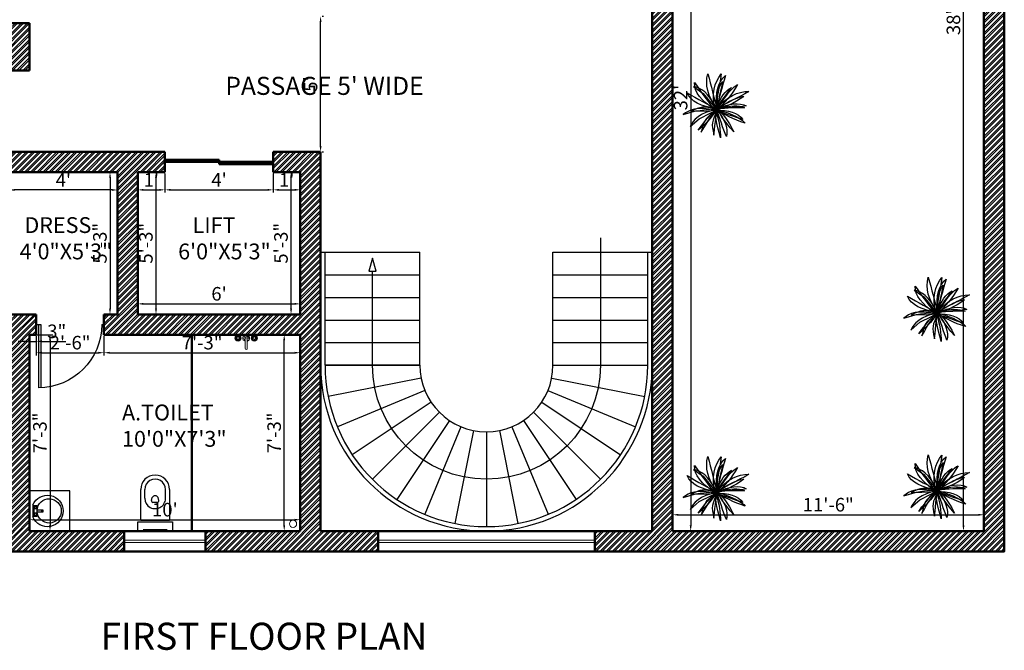
# Model space of a CAD drawing. Units: inches. Extents: x 3590 to 5167, y 65 to 1917.
# Tile 11 of 100: x 4644 to 5080, y 65 to 345. Entities that reach past the tile are written whole.
import ezdxf

# ---------------------------------------------------------------- set-up
doc = ezdxf.new("R2010")
doc.units = ezdxf.units.IN
for name, color, linetype, lineweight in [('A-ANNO-DIMS', 2, 'Continuous', 18), ('A-ANNO-TEXT', 7, 'Continuous', 25), ('A-AREA-IDEN', 7, 'Continuous', 18), ('A-DOOR', 3, 'Continuous', 25), ('A-FLOR-FIXT', 8, 'Continuous', 18), ('A-FLOR-STRS', 7, 'Continuous', 25), ('A-GLAZ', 4, 'Continuous', 18), ('A-WALL', 7, 'Continuous', 50), ('A-WALL-PATT', 251, 'Continuous', 13), ('L-PLNT', 94, 'Continuous', 18)]:
    doc.layers.add(name, color=color, linetype=linetype, lineweight=lineweight)
doc.layers.add('DIENHOA', color=3, linetype='Continuous')
doc.layers.add('SANTEH', color=7, linetype='Continuous')
doc.styles.get("Standard").update_dxf_attribs({"font": 'arial.ttf'})
doc.dimstyles.new('ISO-25', dxfattribs={"dimtxt": 9, "dimasz": 2.5, "dimexe": 1.25, "dimexo": 0.625, "dimtad": 1, "dimdec": 1, "dimlunit": 3, "dimtxsty": 'Standard', "dimcen": 2.5, "dimadec": 0, "dimazin": 0, "dimtfac": 1, "dimtdec": 1, "dimtmove": 0, "dimatfit": 3, "dimfxl": 1, "dimarcsym": 0})

# ---------------------------------------------------------------- blocks, each defined once
blk = doc.blocks.new('*U163')
blk.add_line((-21, 0), (21, 0))
blk = doc.blocks.new('*U162')
at = {"layer": 'A-FLOR-STRS', "color": 0, "linetype": 'ByBlock', "lineweight": -2, "transparency": 16777216}
for p, rotation in [((4076.01, 1459), 89.99999999999982), ((4066.16, 1458.03), 101.2499999999998), ((4085.86, 1458.03), 78.7499999999998), ((4056.69, 1455.15), 112.4999999999998), ((4095.34, 1455.15), 67.4999999999998), ((4047.96, 1450.49), 123.7499999999997), ((4104.07, 1450.49), 56.24999999999984), ((4040.3, 1444.21), 134.9999999999996), ((4111.72, 1444.21), 44.99999999999992), ((4034.02, 1436.56), 146.2499999999996), ((4118, 1436.56), 33.74999999999991), ((4029.36, 1427.82), 157.4999999999995), ((4122.67, 1427.82), 22.49999999999996), ((4026.48, 1418.35), 168.7499999999995), ((4125.54, 1418.35), 11.25), ((4025.51, 1408.5), 180)]:
    blk.add_blockref('*U163', p, dxfattribs=dict(at, rotation=rotation))
blk.add_blockref('*U163', (4126.51, 1408.5), dxfattribs=at)
blk = doc.blocks.new('D2')
for p, q in [((1, 0), (1, 28)), ((2, 0), (2, 27.98)), ((0, 0), (2, 0)), ((29, 0), (30, 0))]:
    blk.add_line(p, q)
at = {"ltscale": 0.5}
blk.add_arc((1, 0), 28, 0, 90, dxfattribs=at)
blk = doc.blocks.new('Cay03_mb')
at = {"layer": 'DIENHOA'}
for p, q in [((79, 504), (119, 555)), ((119, 555), (166, 599)), ((166, 599), (142, 519)), ((-365, 390), (-414, 403)), ((-414, 403), (-240, 278)), ((-315, 371), (-365, 390)), ((-264, 343), (-315, 371)), ((10, 295), (25, 374)), ((25, 374), (49, 444)), ((49, 444), (79, 504)), ((97, 366), (76, 291)), ((119, 442), (97, 366)), ((142, 519), (119, 442)), ((-211, 305), (-264, 343)), ((-240, 278), (-88, 95)), ((-158, 252), (-211, 305)), ((-104, 184), (-158, 252)), ((-50, 98), (-104, 184)), ((0, 105), (2, 206)), ((2, 206), (10, 295)), ((56, 216), (37, 142)), ((76, 291), (56, 216)), ((147, 144), (219, 200)), ((219, 200), (291, 243)), ((364, 193), (290, 155)), ((291, 243), (363, 275)), ((363, 275), (437, 297)), ((438, 231), (364, 193)), ((437, 297), (511, 310)), ((512, 271), (438, 231)), ((511, 310), (586, 314)), ((586, 314), (512, 271)), ((-345, 5), (-400, -17)), ((-299, 20), (-345, 5)), ((-255, 27), (-299, 20)), ((-208, 28), (-255, 27)), ((-153, 22), (-208, 28)), ((-83, 10), (-153, 22)), ((-88, 95), (5, -8)), ((5, -8), (-83, 10)), ((5, -8), (-50, 98)), ((5, -8), (0, 105)), ((5, -8), (76, 75)), ((20, 68), (5, -8)), ((75, 36), (5, -8)), ((5, -8), (100, 18)), ((46, 1), (5, -8)), ((37, 142), (20, 68)), ((97, 7), (46, 1)), ((145, 77), (75, 36)), ((76, 75), (147, 144)), ((155, 12), (97, 7)), ((100, 18), (182, 37)), ((217, 117), (145, 77)), ((220, 15), (155, 12)), ((182, 37), (253, 49)), ((290, 155), (217, 117)), ((289, 17), (220, 15)), ((253, 49), (315, 54)), ((362, 19), (289, 17)), ((315, 54), (369, 53)), ((436, 19), (362, 19)), ((369, 53), (419, 47)), ((419, 47), (465, 35)), ((510, 19), (436, 19)), ((465, 35), (510, 19)), ((-400, -17), (-468, -48)), ((-468, -48), (-376, -38)), ((-376, -38), (-295, -28)), ((-295, -28), (-226, -19)), ((-226, -19), (-166, -11)), ((-216, -236), (-166, -174)), ((-166, -11), (-114, -6)), ((-166, -174), (-120, -122)), ((-120, -122), (-80, -80)), ((-75, -127), (-118, -181)), ((-114, -6), (-69, -3)), ((-80, -80), (-45, -46)), ((-33, -69), (-75, -127)), ((-69, -3), (-30, -3)), ((-45, -46), (-17, -22)), ((5, -8), (-33, -69)), ((-30, -3), (5, -8)), ((-17, -22), (5, -8)), ((5, -8), (57, -73)), ((26, -64), (5, -8)), ((5, -8), (113, -40)), ((53, -42), (5, -8)), ((47, -126), (26, -64)), ((69, -191), (47, -126)), ((107, -76), (53, -42)), ((57, -73), (100, -139)), ((100, -139), (136, -204)), ((166, -110), (107, -76)), ((113, -40), (207, -74)), ((229, -143), (166, -110)), ((207, -74), (290, -108)), ((296, -175), (229, -143)), ((290, -108), (359, -141)), ((367, -205), (296, -175)), ((359, -141), (417, -174)), ((417, -174), (463, -204)), ((-330, -387), (-271, -307)), ((-291, -355), (-330, -387)), ((-250, -318), (-291, -355)), ((-271, -307), (-216, -236)), ((-206, -276), (-250, -318)), ((-162, -231), (-206, -276)), ((-118, -181), (-162, -231)), ((91, -257), (69, -191)), ((113, -322), (91, -257)), ((135, -386), (113, -322)), ((136, -204), (163, -268)), ((163, -268), (181, -330)), ((181, -330), (190, -390)), ((442, -233), (367, -205)), ((519, -258), (442, -233)), ((463, -204), (496, -232)), ((496, -232), (519, -258)), ((158, -445), (135, -386)), ((180, -499), (158, -445)), ((190, -446), (180, -499)), ((190, -390), (190, -446))]:
    blk.add_line(p, q, dxfattribs=at)
for points in [[(24, -5), (-41, 82), (-92, 167), (-130, 249), (-156, 330), (-170, 408), (-175, 484), (-170, 559), (-157, 633)], [(-157, 633), (-132, 551), (-111, 470), (-90, 389), (-70, 309), (-49, 229), (-27, 150), (-3, 72), (24, -5)], [(-16, -27), (-38, 80), (-49, 178), (-49, 269), (-39, 353), (-19, 430), (9, 501), (45, 567), (88, 629)], [(88, 629), (75, 544), (61, 461), (46, 379), (31, 298), (16, 217), (3, 136), (-8, 55), (-16, -27)], [(-396, 474), (-348, 406), (-301, 339), (-254, 275), (-208, 212), (-162, 151), (-115, 91), (-66, 32), (-16, -27)], [(-16, -27), (-108, 39), (-187, 102), (-252, 163), (-305, 224), (-345, 285), (-374, 347), (-390, 409), (-396, 474)], [(273, 387), (228, 329), (182, 270), (138, 212), (97, 156), (60, 103), (28, 55), (2, 11), (-16, -27)], [(-16, -27), (21, 64), (57, 140), (91, 203), (125, 255), (160, 297), (195, 332), (233, 362), (273, 387)], [(24, -5), (20, 93), (20, 177), (25, 249), (34, 310), (47, 363), (65, 409), (87, 452), (113, 492)], [(113, 492), (96, 420), (79, 347), (64, 276), (50, 208), (38, 145), (30, 87), (25, 36), (24, -5)], [(384, 437), (342, 368), (298, 302), (253, 239), (206, 181), (159, 127), (113, 78), (68, 34), (24, -5)], [(24, -5), (80, 92), (134, 176), (186, 248), (234, 309), (279, 357), (319, 395), (355, 421), (384, 437)], [(-530, 290), (-458, 248), (-388, 208), (-319, 169), (-251, 131), (-183, 95), (-115, 60), (-46, 26), (24, -5)], [(24, -5), (-87, 15), (-185, 40), (-270, 68), (-344, 101), (-406, 140), (-457, 184), (-499, 233), (-530, 290)], [(497, 224), (429, 178), (362, 137), (294, 99), (227, 66), (162, 37), (100, 11), (40, -10), (-16, -27)], [(-16, -27), (75, 38), (160, 92), (237, 136), (307, 170), (368, 195), (420, 213), (463, 222), (497, 224)], [(-16, -27), (-134, -5), (-235, 5), (-322, 5), (-396, -5), (-459, -22), (-512, -46), (-558, -74), (-598, -105)], [(24, -5), (99, 30), (173, 57), (245, 77), (313, 88), (378, 92), (438, 87), (493, 74), (541, 52)], [(541, 52), (484, 43), (421, 35), (354, 28), (285, 21), (216, 14), (148, 8), (83, 2), (24, -5)], [(-598, -105), (-393, -44), (-155, -37), (-16, -27)], [(-472, -320), (-310, -179), (-98, -73), (24, -5)], [(24, -5), (-92, -35), (-188, -68), (-267, -105), (-330, -145), (-380, -187), (-418, -231), (-448, -275), (-472, -320)], [(-276, -424), (-227, -345), (-186, -276), (-150, -216), (-119, -164), (-91, -120), (-66, -82), (-41, -52), (-16, -27)], [(-16, -27), (-85, -86), (-137, -133), (-176, -173), (-204, -210), (-226, -249), (-243, -295), (-258, -352), (-276, -424)], [(24, -5), (-14, -88), (-41, -153), (-60, -205), (-70, -251), (-73, -295), (-69, -344), (-60, -402), (-45, -475)], [(-45, -475), (-34, -383), (-25, -303), (-18, -233), (-12, -173), (-6, -121), (2, -77), (11, -39), (24, -5)], [(76, -524), (49, -428), (27, -342), (9, -264), (-4, -196), (-12, -138), (-17, -90), (-18, -53), (-16, -27)], [(478, -192), (422, -176), (361, -157), (298, -135), (232, -113), (167, -89), (102, -67), (41, -45), (-16, -27)], [(-16, -27), (67, -27), (146, -33), (219, -45), (286, -63), (346, -87), (398, -117), (443, -152), (478, -192)], [(-16, -27), (8, -95), (29, -163), (44, -231), (56, -296), (65, -359), (71, -419), (74, -474), (76, -524)], [(316, -418), (251, -343), (195, -273), (147, -210), (106, -154), (74, -105), (50, -63), (33, -30), (24, -5)], [(24, -5), (75, -57), (122, -111), (164, -165), (203, -219), (237, -273), (267, -324), (294, -373), (316, -418)]]:
    blk.add_lwpolyline(points, dxfattribs=at)
blk = doc.blocks.new('*D179')
at = {"layer": 'A-ANNO-DIMS', "color": 0, "lineweight": -2, "transparency": 16777216}
for p, q in [((4639.27, 276.43), (4639.27, 267.91)), ((4687.27, 276.43), (4687.27, 267.91)), ((4684.77, 269.16), (4641.77, 269.16))]:
    blk.add_line(p, q, dxfattribs=at)
at = {"layer": 'A-ANNO-DIMS', "color": 0, "transparency": 16777216}
for points in [[(4641.77, 269.57), (4641.77, 268.74), (4639.27, 269.16)], [(4684.77, 269.57), (4684.77, 268.74), (4687.27, 269.16)]]:
    blk.add_solid(points, dxfattribs=at)
at = {"layer": 'Defpoints', "color": 0, "transparency": 16777216}
for p in [(4639.27, 277.06), (4687.27, 277.06), (4639.27, 269.16)]:
    blk.add_point(p, dxfattribs=at)
at = {"layer": 'A-ANNO-DIMS', "color": 0, "transparency": 16777216, "insert": (4663.27, 272.78), "char_height": 6, "attachment_point": 5}
blk.add_mtext("4'", dxfattribs=at)
blk = doc.blocks.new('*D180')
at = {"layer": 'A-ANNO-DIMS', "color": 0, "lineweight": -2, "transparency": 16777216}
for p, q in [((4686.65, 277.06), (4682.7, 277.06)), ((4683.95, 274.56), (4683.95, 216.56)), ((4686.65, 214.06), (4682.7, 214.06))]:
    blk.add_line(p, q, dxfattribs=at)
at = {"layer": 'A-ANNO-DIMS', "color": 0, "transparency": 16777216}
for points in [[(4683.54, 274.56), (4684.37, 274.56), (4683.95, 277.06)], [(4683.54, 216.56), (4684.37, 216.56), (4683.95, 214.06)]]:
    blk.add_solid(points, dxfattribs=at)
at = {"layer": 'Defpoints', "color": 0, "transparency": 16777216}
for p in [(4687.27, 277.06), (4683.95, 214.06), (4687.27, 214.06)]:
    blk.add_point(p, dxfattribs=at)
at = {"layer": 'A-ANNO-DIMS', "color": 0, "transparency": 16777216, "insert": (4680.26, 245.56), "char_height": 6, "attachment_point": 5, "rotation": 90}
blk.add_mtext('5\'-3"', dxfattribs=at)
blk = doc.blocks.new('*D257')
at = {"layer": 'A-ANNO-DIMS', "color": 0, "lineweight": -2, "transparency": 16777216}
for p, q in [((4645.77, 202.08), (4643.27, 202.08)), ((4648.27, 204.43), (4648.27, 200.83)), ((4648.27, 202.08), (4651.27, 202.08)), ((4651.27, 204.43), (4651.27, 200.83)), ((4653.77, 202.08), (4664.42, 202.08))]:
    blk.add_line(p, q, dxfattribs=at)
at = {"layer": 'A-ANNO-DIMS', "color": 0, "transparency": 16777216}
for points in [[(4645.77, 202.49), (4645.77, 201.66), (4648.27, 202.08)], [(4653.77, 202.49), (4653.77, 201.66), (4651.27, 202.08)]]:
    blk.add_solid(points, dxfattribs=at)
at = {"layer": 'Defpoints', "color": 0, "transparency": 16777216}
for p in [(4648.27, 205.06), (4651.27, 205.06), (4651.27, 202.08)]:
    blk.add_point(p, dxfattribs=at)
at = {"layer": 'A-ANNO-DIMS', "color": 0, "transparency": 16777216, "insert": (4660.35, 205.77), "char_height": 6, "attachment_point": 5}
blk.add_mtext('3"', dxfattribs=at)
blk = doc.blocks.new('*D258')
at = {"layer": 'A-ANNO-DIMS', "color": 0, "lineweight": -2, "transparency": 16777216}
for p, q in [((4651.27, 204.43), (4651.27, 195.81)), ((4681.27, 204.43), (4681.27, 195.81)), ((4653.77, 197.06), (4678.77, 197.06))]:
    blk.add_line(p, q, dxfattribs=at)
at = {"layer": 'A-ANNO-DIMS', "color": 0, "transparency": 16777216}
for points in [[(4653.77, 197.48), (4653.77, 196.65), (4651.27, 197.06)], [(4678.77, 197.48), (4678.77, 196.65), (4681.27, 197.06)]]:
    blk.add_solid(points, dxfattribs=at)
at = {"layer": 'Defpoints', "color": 0, "transparency": 16777216}
for p in [(4651.27, 205.06), (4681.27, 205.06), (4681.27, 197.06)]:
    blk.add_point(p, dxfattribs=at)
at = {"layer": 'A-ANNO-DIMS', "color": 0, "transparency": 16777216, "insert": (4666.27, 200.75), "char_height": 6, "attachment_point": 5}
blk.add_mtext('2\'-6"', dxfattribs=at)
blk = doc.blocks.new('*D259')
at = {"layer": 'A-ANNO-DIMS', "color": 0, "lineweight": -2, "transparency": 16777216}
for p, q in [((4681.27, 204.43), (4681.27, 195.81)), ((4768.27, 204.43), (4768.27, 195.81)), ((4683.77, 197.06), (4765.77, 197.06))]:
    blk.add_line(p, q, dxfattribs=at)
at = {"layer": 'A-ANNO-DIMS', "color": 0, "transparency": 16777216}
for points in [[(4683.77, 197.48), (4683.77, 196.65), (4681.27, 197.06)], [(4765.77, 197.48), (4765.77, 196.65), (4768.27, 197.06)]]:
    blk.add_solid(points, dxfattribs=at)
at = {"layer": 'Defpoints', "color": 0, "transparency": 16777216}
for p in [(4681.27, 205.06), (4768.27, 205.06), (4768.27, 197.06)]:
    blk.add_point(p, dxfattribs=at)
at = {"layer": 'A-ANNO-DIMS', "color": 0, "transparency": 16777216, "insert": (4724.77, 200.75), "char_height": 6, "attachment_point": 5}
blk.add_mtext('7\'-3"', dxfattribs=at)
blk = doc.blocks.new('*D260')
at = {"layer": 'A-ANNO-DIMS', "color": 0, "lineweight": -2, "transparency": 16777216}
for p, q in [((4648.9, 205.06), (4658.62, 205.06)), ((4657.37, 202.56), (4657.37, 120.56)), ((4648.9, 118.06), (4658.62, 118.06))]:
    blk.add_line(p, q, dxfattribs=at)
at = {"layer": 'A-ANNO-DIMS', "color": 0, "transparency": 16777216}
for points in [[(4656.95, 202.56), (4657.78, 202.56), (4657.37, 205.06)], [(4656.95, 120.56), (4657.78, 120.56), (4657.37, 118.06)]]:
    blk.add_solid(points, dxfattribs=at)
at = {"layer": 'Defpoints', "color": 0, "transparency": 16777216}
for p in [(4648.27, 205.06), (4648.27, 118.06), (4657.37, 118.06)]:
    blk.add_point(p, dxfattribs=at)
at = {"layer": 'A-ANNO-DIMS', "color": 0, "transparency": 16777216, "insert": (4653.68, 161.56), "char_height": 6, "attachment_point": 5, "rotation": 90}
blk.add_mtext('7\'-3"', dxfattribs=at)
blk = doc.blocks.new('*D217')
at = {"layer": 'A-ANNO-DIMS', "color": 0, "lineweight": -2, "transparency": 16777216}
for p, q in [((4648.27, 118.68), (4648.27, 124.35)), ((4650.77, 123.1), (4765.77, 123.1)), ((4768.27, 118.68), (4768.27, 124.35))]:
    blk.add_line(p, q, dxfattribs=at)
at = {"layer": 'A-ANNO-DIMS', "color": 0, "transparency": 16777216}
for points in [[(4650.77, 123.52), (4650.77, 122.69), (4648.27, 123.1)], [(4765.77, 123.52), (4765.77, 122.69), (4768.27, 123.1)]]:
    blk.add_solid(points, dxfattribs=at)
at = {"layer": 'Defpoints', "color": 0, "transparency": 16777216}
for p in [(4768.27, 123.1), (4648.27, 118.06), (4768.27, 118.06)]:
    blk.add_point(p, dxfattribs=at)
at = {"layer": 'A-ANNO-DIMS', "color": 0, "transparency": 16777216, "insert": (4708.27, 126.79), "char_height": 6, "attachment_point": 5}
blk.add_mtext("10'", dxfattribs=at)
blk = doc.blocks.new('*D166')
at = {"layer": 'A-ANNO-DIMS', "color": 0, "lineweight": -2, "transparency": 16777216}
for p, q in [((4767.65, 205.06), (4759.91, 205.06)), ((4761.16, 120.56), (4761.16, 202.56)), ((4767.65, 118.06), (4759.91, 118.06))]:
    blk.add_line(p, q, dxfattribs=at)
at = {"layer": 'A-ANNO-DIMS', "color": 0, "transparency": 16777216}
for points in [[(4760.74, 202.56), (4761.57, 202.56), (4761.16, 205.06)], [(4760.74, 120.56), (4761.57, 120.56), (4761.16, 118.06)]]:
    blk.add_solid(points, dxfattribs=at)
at = {"layer": 'Defpoints', "color": 0, "transparency": 16777216}
for p in [(4761.16, 205.06), (4768.27, 205.06), (4768.27, 118.06)]:
    blk.add_point(p, dxfattribs=at)
at = {"layer": 'A-ANNO-DIMS', "color": 0, "transparency": 16777216, "insert": (4757.47, 161.56), "char_height": 6, "attachment_point": 5, "rotation": 90}
blk.add_mtext('7\'-3"', dxfattribs=at)
blk = doc.blocks.new('*D218')
at = {"layer": 'A-ANNO-DIMS', "color": 0, "lineweight": -2, "transparency": 16777216}
for p, q in [((4696.9, 277.06), (4705.58, 277.06)), ((4704.33, 274.56), (4704.33, 216.56)), ((4696.9, 214.06), (4705.58, 214.06))]:
    blk.add_line(p, q, dxfattribs=at)
at = {"layer": 'A-ANNO-DIMS', "color": 0, "transparency": 16777216}
for points in [[(4703.91, 274.56), (4704.74, 274.56), (4704.33, 277.06)], [(4703.91, 216.56), (4704.74, 216.56), (4704.33, 214.06)]]:
    blk.add_solid(points, dxfattribs=at)
at = {"layer": 'Defpoints', "color": 0, "transparency": 16777216}
for p in [(4696.27, 277.06), (4696.27, 214.06), (4704.33, 214.06)]:
    blk.add_point(p, dxfattribs=at)
at = {"layer": 'A-ANNO-DIMS', "color": 0, "transparency": 16777216, "insert": (4700.63, 245.56), "char_height": 6, "attachment_point": 5, "rotation": 90}
blk.add_mtext('5\'-3"', dxfattribs=at)
blk = doc.blocks.new('*D219')
at = {"layer": 'A-ANNO-DIMS', "color": 0, "lineweight": -2, "transparency": 16777216}
for p, q in [((4696.27, 214.68), (4696.27, 219.95)), ((4698.77, 218.7), (4765.77, 218.7)), ((4768.27, 214.68), (4768.27, 219.95))]:
    blk.add_line(p, q, dxfattribs=at)
at = {"layer": 'A-ANNO-DIMS', "color": 0, "transparency": 16777216}
for points in [[(4698.77, 219.12), (4698.77, 218.29), (4696.27, 218.7)], [(4765.77, 219.12), (4765.77, 218.29), (4768.27, 218.7)]]:
    blk.add_solid(points, dxfattribs=at)
at = {"layer": 'Defpoints', "color": 0, "transparency": 16777216}
for p in [(4768.27, 218.7), (4696.27, 214.06), (4768.27, 214.06)]:
    blk.add_point(p, dxfattribs=at)
at = {"layer": 'A-ANNO-DIMS', "color": 0, "transparency": 16777216, "insert": (4732.27, 222.39), "char_height": 6, "attachment_point": 5}
blk.add_mtext("6'", dxfattribs=at)
blk = doc.blocks.new('*D220')
at = {"layer": 'A-ANNO-DIMS', "color": 0, "lineweight": -2, "transparency": 16777216}
for p, q in [((4767.65, 277.06), (4762.93, 277.06)), ((4764.18, 216.56), (4764.18, 274.56)), ((4767.65, 214.06), (4762.93, 214.06))]:
    blk.add_line(p, q, dxfattribs=at)
at = {"layer": 'A-ANNO-DIMS', "color": 0, "transparency": 16777216}
for points in [[(4763.77, 274.56), (4764.6, 274.56), (4764.18, 277.06)], [(4763.77, 216.56), (4764.6, 216.56), (4764.18, 214.06)]]:
    blk.add_solid(points, dxfattribs=at)
at = {"layer": 'Defpoints', "color": 0, "transparency": 16777216}
for p in [(4764.18, 277.06), (4768.27, 277.06), (4768.27, 214.06)]:
    blk.add_point(p, dxfattribs=at)
at = {"layer": 'A-ANNO-DIMS', "color": 0, "transparency": 16777216, "insert": (4760.49, 245.56), "char_height": 6, "attachment_point": 5, "rotation": 90}
blk.add_mtext('5\'-3"', dxfattribs=at)
blk = doc.blocks.new('*D221')
at = {"layer": 'A-ANNO-DIMS', "color": 0, "lineweight": -2, "transparency": 16777216}
for p, q in [((4696.27, 276.43), (4696.27, 267.96)), ((4708.27, 276.43), (4708.27, 267.96)), ((4698.77, 269.21), (4705.77, 269.21))]:
    blk.add_line(p, q, dxfattribs=at)
at = {"layer": 'A-ANNO-DIMS', "color": 0, "transparency": 16777216}
for points in [[(4698.77, 269.62), (4698.77, 268.79), (4696.27, 269.21)], [(4705.77, 269.62), (4705.77, 268.79), (4708.27, 269.21)]]:
    blk.add_solid(points, dxfattribs=at)
at = {"layer": 'Defpoints', "color": 0, "transparency": 16777216}
for p in [(4696.27, 277.06), (4708.27, 277.06), (4708.27, 269.21)]:
    blk.add_point(p, dxfattribs=at)
at = {"layer": 'A-ANNO-DIMS', "color": 0, "transparency": 16777216, "insert": (4702.27, 272.84), "char_height": 6, "attachment_point": 5}
blk.add_mtext("1'", dxfattribs=at)
blk = doc.blocks.new('*D253')
at = {"layer": 'A-ANNO-DIMS', "color": 0, "lineweight": -2, "transparency": 16777216}
for p, q in [((4708.27, 276.43), (4708.27, 267.96)), ((4756.27, 276.43), (4756.27, 267.96)), ((4710.77, 269.21), (4753.77, 269.21))]:
    blk.add_line(p, q, dxfattribs=at)
at = {"layer": 'A-ANNO-DIMS', "color": 0, "transparency": 16777216}
for points in [[(4710.77, 269.62), (4710.77, 268.79), (4708.27, 269.21)], [(4753.77, 269.62), (4753.77, 268.79), (4756.27, 269.21)]]:
    blk.add_solid(points, dxfattribs=at)
at = {"layer": 'Defpoints', "color": 0, "transparency": 16777216}
for p in [(4708.27, 277.06), (4756.27, 277.06), (4756.27, 269.21)]:
    blk.add_point(p, dxfattribs=at)
at = {"layer": 'A-ANNO-DIMS', "color": 0, "transparency": 16777216, "insert": (4732.27, 272.83), "char_height": 6, "attachment_point": 5}
blk.add_mtext("4'", dxfattribs=at)
blk = doc.blocks.new('*D254')
at = {"layer": 'A-ANNO-DIMS', "color": 0, "lineweight": -2, "transparency": 16777216}
for p, q in [((4756.27, 276.43), (4756.27, 267.96)), ((4768.27, 276.43), (4768.27, 267.96)), ((4758.77, 269.21), (4765.77, 269.21))]:
    blk.add_line(p, q, dxfattribs=at)
at = {"layer": 'A-ANNO-DIMS', "color": 0, "transparency": 16777216}
for points in [[(4758.77, 269.62), (4758.77, 268.79), (4756.27, 269.21)], [(4765.77, 269.62), (4765.77, 268.79), (4768.27, 269.21)]]:
    blk.add_solid(points, dxfattribs=at)
at = {"layer": 'Defpoints', "color": 0, "transparency": 16777216}
for p in [(4756.27, 277.06), (4768.27, 277.06), (4768.27, 269.21)]:
    blk.add_point(p, dxfattribs=at)
at = {"layer": 'A-ANNO-DIMS', "color": 0, "transparency": 16777216, "insert": (4762.27, 272.84), "char_height": 6, "attachment_point": 5}
blk.add_mtext("1'", dxfattribs=at)
blk = doc.blocks.new('*D255')
at = {"layer": 'A-ANNO-DIMS', "color": 0, "lineweight": -2, "transparency": 16777216}
for p, q in [((4933.27, 118.68), (4933.27, 126.54)), ((4935.77, 125.29), (5068.77, 125.29)), ((5071.27, 118.68), (5071.27, 126.54))]:
    blk.add_line(p, q, dxfattribs=at)
at = {"layer": 'A-ANNO-DIMS', "color": 0, "transparency": 16777216}
for points in [[(4935.77, 125.71), (4935.77, 124.87), (4933.27, 125.29)], [(5068.77, 125.71), (5068.77, 124.87), (5071.27, 125.29)]]:
    blk.add_solid(points, dxfattribs=at)
at = {"layer": 'Defpoints', "color": 0, "transparency": 16777216}
for p in [(5071.27, 125.29), (4933.27, 118.06), (5071.27, 118.06)]:
    blk.add_point(p, dxfattribs=at)
at = {"layer": 'A-ANNO-DIMS', "color": 0, "transparency": 16777216, "insert": (5002.27, 128.98), "char_height": 6, "attachment_point": 5}
blk.add_mtext('11\'-6"', dxfattribs=at)
blk = doc.blocks.new('*D256')
at = {"layer": 'A-ANNO-DIMS', "color": 0, "lineweight": -2, "transparency": 16777216}
for p, q in [((5070.65, 580.06), (5060.93, 580.06)), ((5062.18, 120.56), (5062.18, 577.56)), ((5070.65, 118.06), (5060.93, 118.06))]:
    blk.add_line(p, q, dxfattribs=at)
at = {"layer": 'A-ANNO-DIMS', "color": 0, "transparency": 16777216}
for points in [[(5061.77, 577.56), (5062.6, 577.56), (5062.18, 580.06)], [(5061.77, 120.56), (5062.6, 120.56), (5062.18, 118.06)]]:
    blk.add_solid(points, dxfattribs=at)
at = {"layer": 'Defpoints', "color": 0, "transparency": 16777216}
for p in [(5062.18, 580.06), (5071.27, 580.06), (5071.27, 118.06)]:
    blk.add_point(p, dxfattribs=at)
at = {"layer": 'A-ANNO-DIMS', "color": 0, "transparency": 16777216, "insert": (5058.49, 349.06), "char_height": 6, "attachment_point": 5, "rotation": 90}
blk.add_mtext('38\'-6"', dxfattribs=at)
blk = doc.blocks.new('*D236')
at = {"layer": 'A-ANNO-DIMS', "color": 0, "lineweight": -2, "transparency": 16777216}
for p, q in [((4933.9, 502.06), (4942.54, 502.06)), ((4941.29, 499.56), (4941.29, 120.56)), ((4933.9, 118.06), (4942.54, 118.06))]:
    blk.add_line(p, q, dxfattribs=at)
at = {"layer": 'A-ANNO-DIMS', "color": 0, "transparency": 16777216}
for points in [[(4940.87, 499.56), (4941.71, 499.56), (4941.29, 502.06)], [(4940.87, 120.56), (4941.71, 120.56), (4941.29, 118.06)]]:
    blk.add_solid(points, dxfattribs=at)
at = {"layer": 'Defpoints', "color": 0, "transparency": 16777216}
for p in [(4933.27, 502.06), (4933.27, 118.06), (4941.29, 118.06)]:
    blk.add_point(p, dxfattribs=at)
at = {"layer": 'A-ANNO-DIMS', "color": 0, "transparency": 16777216, "insert": (4937.6, 310.06), "char_height": 6, "attachment_point": 5, "rotation": 90}
blk.add_mtext("32'", dxfattribs=at)
blk = doc.blocks.new('*D231')
at = {"layer": 'A-ANNO-DIMS', "color": 0, "lineweight": -2, "transparency": 16777216}
for p, q in [((4777.9, 346.06), (4778.52, 346.06)), ((4777.27, 288.56), (4777.27, 343.56)), ((4777.9, 286.06), (4778.52, 286.06))]:
    blk.add_line(p, q, dxfattribs=at)
at = {"layer": 'A-ANNO-DIMS', "color": 0, "transparency": 16777216}
for points in [[(4776.86, 343.56), (4777.69, 343.56), (4777.27, 346.06)], [(4776.86, 288.56), (4777.69, 288.56), (4777.27, 286.06)]]:
    blk.add_solid(points, dxfattribs=at)
at = {"layer": 'Defpoints', "color": 0, "transparency": 16777216}
for p in [(4777.27, 346.06), (4777.27, 346.06), (4777.27, 286.06)]:
    blk.add_point(p, dxfattribs=at)
at = {"layer": 'A-ANNO-DIMS', "color": 0, "transparency": 16777216, "insert": (4773.6, 316.06), "char_height": 6, "attachment_point": 5, "rotation": 90}
blk.add_mtext("5'", dxfattribs=at)
blk = doc.blocks.new('y3')
at = {"layer": 'SANTEH', "ltscale": 5}
for p, q in [((38, 131), (38, 521)), ((88, 411), (88, 521)), ((347, 426), (348, 521)), ((398, 521), (398, 131)), ((172, 385), (181, 421)), ((263, 385), (254, 421)), ((244, 358), (191, 358)), ((398, 131), (38, 131)), ((67, 21), (367, 21))]:
    blk.add_line(p, q, dxfattribs=at)
blk.add_lwpolyline([(0, 115), (435, 115), (435, 0), (0, 0), (0, 115)], dxfattribs=at)
for centre, radius, start, end in [((218, 521), 180, 0, 180), ((218, 521), 130, 359.1579, 180), ((218, 411), 130, 180, 5.9855), ((191, 378), 20, 160.5038, 270), ((218, 400), 42.2, 30.5234, 149.4766), ((244, 378), 20, 270, 19.4962)]:
    blk.add_arc(centre, radius, start, end, dxfattribs=at)
blk = doc.blocks.new('r11')
at = {"layer": 'SANTEH', "ltscale": 5}
for p, q in [((0, 0), (600, 0)), ((0, -600), (0, 0)), ((600, 0), (600, -600)), ((210, -50), (390, -50)), ((210, -50), (210, -50)), ((224, -63), (376, -63)), ((224, -113), (224, -63)), ((376, -113), (224, -113)), ((233, -79), (249, -69)), ((233, -98), (233, -79)), ((249, -107), (233, -98)), ((249, -69), (266, -79)), ((266, -98), (249, -107)), ((266, -79), (266, -98)), ((288, -202), (288, -113)), ((312, -113), (312, -202)), ((334, -79), (351, -69)), ((334, -98), (334, -79)), ((351, -107), (334, -98)), ((351, -69), (367, -79)), ((367, -98), (351, -107)), ((367, -79), (367, -98)), ((376, -63), (376, -113)), ((312, -184), (288, -184)), ((312, -202), (288, -202)), ((600, -600), (0, -600))]:
    blk.add_line(p, q, dxfattribs=at)
for centre, radius, start, end in [((300, -266), 234, 112.5, 67.5), ((300, -293), 180, 93.8183, 86.1817)]:
    blk.add_arc(centre, radius, start, end, dxfattribs=at)
blk = doc.blocks.new('Faucet - Bathroom top')
for p, q in [((-4.107, 0.125), (-4.375, 0.125)), ((-3.75, 0.4788), (-3.75, 0.75)), ((-3.5, 0.482), (-3.5, 0.75)), ((-3.1461, 0.125), (-2.875, 0.125)), ((3.143, 0.125), (2.875, 0.125)), ((3.5, 0.4788), (3.5, 0.75)), ((3.75, 0.482), (3.75, 0.75)), ((4.1039, 0.125), (4.375, 0.125)), ((-4.1039, -0.125), (-4.375, -0.125)), ((-3.75, -0.4821), (-3.75, -0.75)), ((-3.5, -0.4789), (-3.5, -0.75)), ((-3.143, -0.125), (-2.875, -0.125)), ((-0.5, -0.8639), (-0.5, -4.5)), ((0.5, -4.5), (0.5, -0.8631)), ((3.1461, -0.125), (2.875, -0.125)), ((3.5, -0.4821), (3.5, -0.75)), ((3.75, -0.4789), (3.75, -0.75)), ((4.107, -0.125), (4.375, -0.125))]:
    blk.add_line(p, q)
for centre, radius in [((-3.625, 0), 1.375), ((-4.625, 0), 0.2795), ((-3.625, 0), 0.5), ((-3.625, 1), 0.2795), ((-2.625, 0), 0.2795), ((0, 0), 0.5), ((3.625, 0), 1.375), ((2.625, 0), 0.2795), ((3.625, 0), 0.5), ((3.625, 1), 0.2795), ((4.625, 0), 0.2795), ((-3.625, -1), 0.2795), ((3.625, -1), 0.2795)]:
    blk.add_circle(centre, radius)
for centre, radius, start, end in [((-3.625, 0), 1, 105.2407, 164.2093), ((-3.625, 0), 1, 16.44125, 74.07887), ((0, 0), 1.5, 289.6514, 250.3603), ((0, 0), 1, 300.3431, 239.7554), ((3.625, 0), 1, 106.12, 164.0884), ((3.625, 0), 1, 16.23422, 73.90469), ((-3.625, 0), 1, 196.2342, 253.9047), ((-3.625, 0), 1, 286.12, 344.0884), ((3.625, 0), 1, 196.4413, 254.0789), ((3.625, 0), 1, 285.2407, 344.2093), ((0, -4.5), 0.5, 180, 0)]:
    blk.add_arc(centre, radius, start, end)

msp = doc.modelspace()

# ---------------------------------------------------------------- hatches: boundary and pattern name
at = {"layer": 'A-WALL-PATT', "transparency": 33554687}
h = msp.add_hatch(dxfattribs=at)
h.set_pattern_fill('ANSI32', color=256, scale=0.2)
h.set_pattern_definition([(45, (0, -1216.9392), (-1.3470384, 1.3470384), []), (45, (0.898, -1216.9392), (-1.3470384, 1.3470384), [])])
h.paths.add_polyline_path([(4684.27, 589.06), (4591.27, 589.06), (4591.27, 580.06), (4639.27, 580.06), (4639.27, 574.06), (4648.27, 574.06), (4648.27, 580.06), (4684.27, 580.06)])
h.paths.add_polyline_path([(4543.27, 589.06), (4420.27, 589.06), (4420.27, 568.06), (4429.27, 568.06), (4429.27, 580.06), (4445.92, 580.06), (4543.27, 580.06)])
h.paths.add_polyline_path([(4828.27, 589.06), (4744.27, 589.06), (4744.27, 580.06), (4828.27, 580.06)])
h.paths.add_polyline_path([(4648.27, 538.06), (4639.27, 538.06), (4639.27, 439.06), (4546.27, 439.06), (4546.27, 433.06), (4549.27, 433.06), (4549.27, 337.06), (4429.27, 337.06), (4429.27, 367.06), (4420.27, 367.06), (4420.27, 322.06), (4429.27, 322.06), (4429.27, 328.06), (4639.27, 328.06), (4639.27, 322.06), (4648.27, 322.06), (4648.27, 343.06), (4639.27, 343.06), (4639.27, 337.06), (4555.27, 337.06), (4555.27, 433.06), (4639.27, 433.06), (4639.27, 373.06), (4648.27, 373.06)])
h.paths.add_polyline_path([(4516.27, 439.06), (4429.27, 439.06), (4429.27, 520.06), (4420.27, 520.06), (4420.27, 403.06), (4429.27, 403.06), (4429.27, 433.06), (4516.27, 433.06)], flags=17)
h.paths.add_polyline_path([(5080.27, 589.06), (4888.27, 589.06), (4888.27, 580.06), (4924.27, 580.06), (4924.27, 538.06), (4933.27, 538.06), (4933.27, 580.06), (5071.27, 580.06), (5071.27, 118.06), (4933.27, 118.06), (4933.27, 349.06), (4924.27, 349.06), (4924.27, 118.06), (4898.77, 118.06), (4898.77, 109.06), (5080.27, 109.06)])
h.paths.add_polyline_path([(4933.27, 502.06), (4924.27, 502.06), (4924.27, 421.06), (4933.27, 421.06)], flags=17)
h.paths.add_polyline_path([(4802.77, 118.06), (4777.27, 118.06), (4777.27, 286.06), (4756.27, 286.06), (4756.27, 277.06), (4768.27, 277.06), (4768.27, 214.06), (4696.27, 214.06), (4696.27, 277.06), (4708.27, 277.06), (4708.27, 286.06), (4639.27, 286.06), (4639.27, 277.06), (4687.27, 277.06), (4687.27, 214.06), (4681.27, 214.06), (4681.27, 205.06), (4768.27, 205.06), (4768.27, 118.06), (4726.27, 118.06), (4726.27, 109.06), (4802.77, 109.06)])
h.paths.add_polyline_path([(4690.27, 118.06), (4648.27, 118.06), (4648.27, 135.93), (4648.27, 205.06), (4651.27, 205.06), (4651.27, 214.06), (4639.27, 214.06), (4639.27, 118.06), (4633.27, 118.06), (4633.27, 109.06), (4690.27, 109.06)])
h.paths.add_polyline_path([(4585.27, 118.06), (4584.72, 118.06), (4429.27, 118.06), (4429.27, 274.06), (4420.27, 274.06), (4420.27, 109.06), (4585.27, 109.06)])

# ---------------------------------------------------------------- linework, layer by layer
at = {"layer": 'A-FLOR-FIXT'}
msp.add_circle((4765.07, 121.27), 1.6, dxfattribs=at)
at = {"layer": 'A-FLOR-STRS'}
for p, q in [((4777.27, 241.56), (4821.27, 241.56)), ((4779.27, 191.56), (4779.27, 241.56)), ((4821.27, 191.56), (4821.27, 241.56)), ((4880.27, 241.56), (4924.27, 241.56)), ((4880.27, 191.56), (4880.27, 241.56)), ((4922.27, 191.56), (4922.27, 241.56)), ((4779.27, 231.56), (4821.27, 231.56)), ((4880.27, 231.56), (4922.27, 231.56)), ((4779.27, 221.56), (4821.27, 221.56)), ((4880.27, 221.56), (4922.27, 221.56)), ((4779.27, 211.56), (4821.27, 211.56)), ((4880.27, 211.56), (4922.27, 211.56)), ((4779.27, 201.56), (4821.27, 201.56)), ((4880.27, 201.56), (4922.27, 201.56)), ((4779.27, 191.56), (4821.27, 191.56))]:
    msp.add_line(p, q, dxfattribs=at)
msp.add_lwpolyline([(4901.27, 248), (4901.27, 191.56, -1), (4800.27, 191.56), (4800.27, 233.17)], format="xyb", dxfattribs=at)
msp.add_lwpolyline([(4800.27, 238.93), (4798.64, 233.17), (4801.91, 233.17)], close=True, dxfattribs=at)
for radius in [73.5, 71.5, 29.5]:
    msp.add_arc((4850.77, 191.56), radius, 180, 0, dxfattribs=at)
at = {"layer": 'A-GLAZ'}
for p, q in [((4726.27, 114.06), (4690.27, 114.06)), ((4898.77, 114.06), (4802.77, 114.06)), ((4726.27, 113.06), (4690.27, 113.06)), ((4898.77, 113.06), (4802.77, 113.06))]:
    msp.add_line(p, q, dxfattribs=at)
at = {"layer": 'A-WALL'}
for p, q in [((5071.27, 118.06), (5071.27, 580.06)), ((4924.27, 118.06), (4924.27, 502.06)), ((4933.27, 118.06), (4933.27, 502.06)), ((4648.27, 343.06), (4639.27, 343.06)), ((4648.27, 322.06), (4648.27, 343.06)), ((4648.27, 322.06), (4639.27, 322.06)), ((4708.27, 286.06), (4639.27, 286.06)), ((4708.27, 277.06), (4708.27, 286.06)), ((4777.27, 286.06), (4756.27, 286.06)), ((4756.27, 277.06), (4756.27, 286.06)), ((4777.27, 118.06), (4777.27, 286.06)), ((4708.27, 282.56), (4732.27, 282.56)), ((4708.27, 281.56), (4756.27, 281.56)), ((4732.27, 282.56), (4732.27, 280.56)), ((4732.27, 280.56), (4756.27, 280.56)), ((4687.27, 277.06), (4639.27, 277.06)), ((4687.27, 214.06), (4687.27, 277.06)), ((4708.27, 277.06), (4696.27, 277.06)), ((4696.27, 214.06), (4696.27, 277.06)), ((4768.27, 277.06), (4756.27, 277.06)), ((4768.27, 214.06), (4768.27, 277.06)), ((4651.27, 214.06), (4639.27, 214.06)), ((4651.27, 205.06), (4651.27, 214.06)), ((4687.27, 214.06), (4681.27, 214.06)), ((4681.27, 205.06), (4681.27, 214.06)), ((4768.27, 214.06), (4696.27, 214.06)), ((4651.27, 205.06), (4648.27, 205.06)), ((4648.27, 118.06), (4648.27, 205.06)), ((4768.27, 205.06), (4681.27, 205.06)), ((4720.27, 118.06), (4720.27, 205.06)), ((4768.27, 118.06), (4768.27, 205.06)), ((4768.27, 118.06), (4648.27, 118.06)), ((4690.27, 118.06), (4690.27, 109.06)), ((4726.27, 118.06), (4726.27, 109.06)), ((4924.27, 118.06), (4777.27, 118.06)), ((4802.77, 118.06), (4802.77, 109.06)), ((4898.77, 118.06), (4898.77, 109.06)), ((5071.27, 118.06), (4933.27, 118.06))]:
    msp.add_line(p, q, dxfattribs=at)
msp.add_lwpolyline([(5080.27, 589.06), (5080.27, 109.06), (4420.27, 109.06), (4420.27, 589.06)], close=True, dxfattribs=at)

# ---------------------------------------------------------------- block references
at = {"layer": 'A-DOOR', "xscale": -1, "rotation": 180}
msp.add_blockref('D2', (4651.27, 209.56), dxfattribs=at)
at = {"layer": 'A-FLOR-FIXT'}
msp.add_blockref('Faucet - Bathroom top', (4744.31, 203.56), dxfattribs=at)
at = {"layer": 'A-FLOR-FIXT', "xscale": 0.0353848906415677, "yscale": 0.0353848906415677, "zscale": 0.0353848906415677}
msp.add_blockref('y3', (4696.24, 118.06), dxfattribs=at)
at = {"layer": 'A-FLOR-FIXT', "xscale": -0.0297800069284724, "yscale": 0.0297800069284724, "zscale": 0.0297800069284724, "rotation": 90}
msp.add_blockref('r11', (4648.27, 135.93), dxfattribs=at)
at = {"layer": 'A-FLOR-STRS', "xscale": -1, "rotation": 180}
msp.add_blockref('*U162', (774.76, 1600.06), dxfattribs=at)
at = {"layer": 'L-PLNT', "xscale": 0.0245452446402784, "yscale": 0.0245452446402784, "zscale": 0.0245452446402784}
for p in [(4952.67, 305.09), (5050.43, 214.95), (4952.67, 135.5), (5050.43, 136.3)]:
    msp.add_blockref('Cay03_mb', p, dxfattribs=at)

# ---------------------------------------------------------------- texts
at = {"layer": 'A-ANNO-TEXT', "insert": (4679.79, 77.49), "char_height": 12, "attachment_point": 1}
msp.add_mtext_dynamic_manual_height_columns('{\\fTimes New Roman|b0|i0|c0|p18;FIRST FLOOR PLAN}', width=197.6934, gutter_width=12.5, heights=[0], dxfattribs=at)
at = {"layer": 'A-AREA-IDEN', "attachment_point": 1}
for s, width, insert, char_height in [("{\\fTimes New Roman|b0|i0|c0|p18;PASSAGE 5' WIDE}", 131.4857, (4735.07, 319.26), 8), ('{\\fTimes New Roman|b0|i0|c0|p18; DRESS\\P4\'0"X5\'3"}', 67.3508, (4643.89, 257.09), 7), ('{\\fTimes New Roman|b0|i0|c0|p18;   LIFT\\P6\'0"X5\'3"}', 67.3508, (4714.15, 257.09), 7), ('{\\fTimes New Roman|b0|i0|c0|p18;A.TOILET\\P10\'0"X7\'3"}', 67.3508, (4689.28, 174.1), 7)]:
    msp.add_mtext_dynamic_manual_height_columns(s, width=width, gutter_width=12.5, heights=[0], dxfattribs=dict(at, insert=insert, char_height=char_height))

# ---------------------------------------------------------------- dimensions: what is measured, and where the dimension line sits
at = {"layer": 'A-ANNO-DIMS'}
for base, p1, p2, override, picture, middle in [((5062.18, 580.06), (5071.27, 118.06), (5071.27, 580.06), {"dimtxt": 6, "dimclrd": 0, "dimclre": 0, "dimclrt": 0}, '*D256', (5058.49, 349.06)), ((4941.29, 118.06), (4933.27, 502.06), (4933.27, 118.06), {"dimtxt": 6, "dimclrd": 0, "dimclre": 0, "dimclrt": 0, "dimtmove": 1}, '*D236', (4937.6, 310.06)), ((4777.27, 346.06), (4777.27, 286.06), (4777.27, 346.06), {"dimtxt": 6, "dimclrd": 0, "dimclre": 0, "dimclrt": 0}, '*D231', (4773.6, 316.06)), ((4683.95, 214.06), (4687.27, 277.06), (4687.27, 214.06), {"dimtxt": 6, "dimclrd": 0, "dimclre": 0, "dimclrt": 0}, '*D180', (4680.26, 245.56)), ((4704.33, 214.06), (4696.27, 277.06), (4696.27, 214.06), {"dimtxt": 6, "dimclrd": 0, "dimclre": 0, "dimclrt": 0}, '*D218', (4700.63, 245.56)), ((4764.18, 277.06), (4768.27, 214.06), (4768.27, 277.06), {"dimtxt": 6, "dimclrd": 0, "dimclre": 0, "dimclrt": 0}, '*D220', (4760.49, 245.56)), ((4657.37, 118.06), (4648.27, 205.06), (4648.27, 118.06), {"dimtxt": 6, "dimclrd": 0, "dimclre": 0, "dimclrt": 0}, '*D260', (4653.68, 161.56)), ((4761.16, 205.06), (4768.27, 118.06), (4768.27, 205.06), {"dimtxt": 6, "dimclrd": 0, "dimclre": 0, "dimclrt": 0}, '*D166', (4757.47, 161.56))]:
    dim = msp.add_linear_dim(base=base, p1=p1, p2=p2, angle=90, dimstyle='ISO-25', override=override, dxfattribs=at)
    dim.commit()
    dim.dimension.update_dxf_attribs({"geometry": picture, "text_midpoint": middle})
for base, p1, p2, override, picture, middle in [((4639.27, 269.16), (4687.27, 277.06), (4639.27, 277.06), {"dimtxt": 6, "dimclrd": 0, "dimclre": 0, "dimclrt": 0}, '*D179', (4663.27, 272.78)), ((4708.27, 269.21), (4696.27, 277.06), (4708.27, 277.06), {"dimtxt": 6, "dimclrd": 0, "dimclre": 0, "dimclrt": 0}, '*D221', (4702.27, 272.84)), ((4756.27, 269.21), (4708.27, 277.06), (4756.27, 277.06), {"dimtxt": 6, "dimclrd": 0, "dimclre": 0, "dimclrt": 0, "dimtmove": 1}, '*D253', (4732.27, 272.83)), ((4768.27, 269.21), (4756.27, 277.06), (4768.27, 277.06), {"dimtxt": 6, "dimclrd": 0, "dimclre": 0, "dimclrt": 0, "dimtmove": 1}, '*D254', (4762.27, 272.84)), ((4768.27, 218.7), (4696.27, 214.06), (4768.27, 214.06), {"dimtxt": 6, "dimclrd": 0, "dimclre": 0, "dimclrt": 0}, '*D219', (4732.27, 222.39)), ((4651.27, 202.08), (4648.27, 205.06), (4651.27, 205.06), {"dimtxt": 6, "dimclrd": 0, "dimclre": 0, "dimclrt": 0}, '*D257', (4660.35, 205.77)), ((4681.27, 197.06), (4651.27, 205.06), (4681.27, 205.06), {"dimtxt": 6, "dimclrd": 0, "dimclre": 0, "dimclrt": 0, "dimtmove": 1}, '*D258', (4666.27, 200.75)), ((4768.27, 197.06), (4681.27, 205.06), (4768.27, 205.06), {"dimtxt": 6, "dimclrd": 0, "dimclre": 0, "dimclrt": 0, "dimtmove": 1}, '*D259', (4724.77, 200.75)), ((5071.27, 125.29), (4933.27, 118.06), (5071.27, 118.06), {"dimtxt": 6, "dimclrd": 0, "dimclre": 0, "dimclrt": 0}, '*D255', (5002.27, 128.98)), ((4768.27, 123.1), (4648.27, 118.06), (4768.27, 118.06), {"dimtxt": 6, "dimclrd": 0, "dimclre": 0, "dimclrt": 0}, '*D217', (4708.27, 126.79))]:
    dim = msp.add_linear_dim(base=base, p1=p1, p2=p2, dimstyle='ISO-25', override=override, dxfattribs=at)
    dim.commit()
    dim.dimension.update_dxf_attribs({"geometry": picture, "text_midpoint": middle})

doc.saveas('drawing.dxf')
